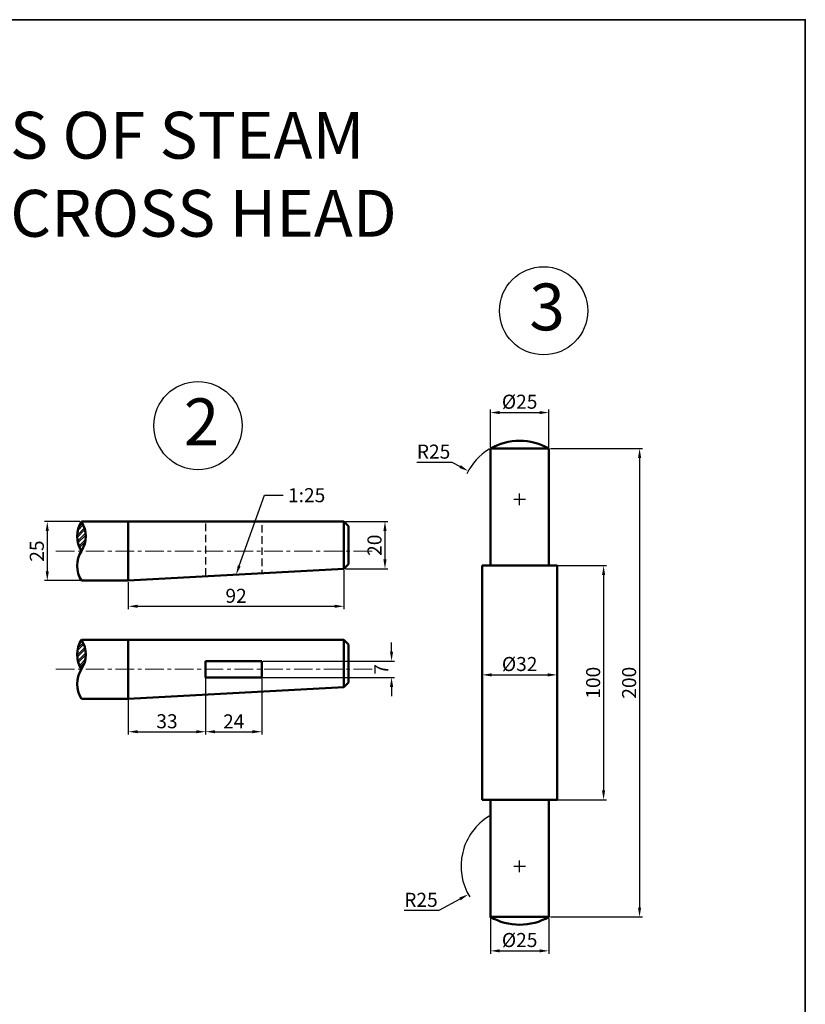
# Model space of a CAD drawing. Units: millimetres. Extents: x 208 to 901, y -26 to 704.
# Tile 3 of 3: x 566 to 901, y 283 to 704. Entities that reach past the tile are written whole.
import ezdxf
from ezdxf import colors
from ezdxf.entities.mleader import LeaderData, LeaderLine
from ezdxf.math import Vec2, Vec3

# ---------------------------------------------------------------- set-up
doc = ezdxf.new("R2010")
doc.units = ezdxf.units.MM
doc.header["$LTSCALE"] = 0.5
doc.linetypes.add('CENTER', pattern=[50.8, 31.75, -6.35, 6.35, -6.35])
doc.linetypes.add('DASHED', pattern=[19.05, 12.7, -6.35])
for name, color, linetype, lineweight in [('M-CNTR', 1, 'CENTER', 18), ('M-DIMS', 2, 'Continuous', 25), ('M-HATC', 8, 'Continuous', 18), ('M-HIDN', 6, 'DASHED', 25), ('M-OUTL', 7, 'Continuous', 50), ('M-TEXT', 3, 'Continuous', 25), ('M-TTLB', 7, 'Continuous', 35)]:
    doc.layers.add(name, color=color, linetype=linetype, lineweight=lineweight)
doc.styles.get("Standard").update_dxf_attribs({"font": 'arial.ttf'})
doc.dimstyles.new('ISO-25', dxfattribs={"dimtxt": 6, "dimasz": 4, "dimexe": 1.25, "dimexo": 0.625, "dimtad": 1, "dimtoh": 1, "dimdec": 0, "dimtxsty": 'Standard', "dimcen": 2.5, "dimadec": 0, "dimazin": 0, "dimtfac": 1, "dimtdec": 0, "dimtofl": 0, "dimtmove": 0, "dimatfit": 3, "dimfxl": 1, "dimarcsym": 0})

# ---------------------------------------------------------------- blocks, each defined once
blk = doc.blocks.new('*D32')
at = {"layer": 'Defpoints', "color": 0, "ltscale": 0.5, "transparency": 16777216}
for p in [(757.07, 510.97), (778.98, 498.94)]:
    blk.add_point(p, dxfattribs=at)
at = {"layer": 'M-DIMS', "color": 0, "lineweight": -2, "ltscale": 0.5, "transparency": 16777216}
for p, q in [((735.05, 514.83), (750.06, 514.83)), ((750.06, 514.83), (753.56, 512.9)), ((778.98, 496.44), (778.98, 501.44)), ((776.48, 498.94), (781.48, 498.94))]:
    blk.add_line(p, q, dxfattribs=at)
blk.add_arc((778.98, 498.94), 25, 121.4324, 154.0897, dxfattribs=at)
at = {"layer": 'M-DIMS', "color": 0, "ltscale": 0.5, "transparency": 16777216}
blk.add_solid([(753.88, 513.48), (753.24, 512.32), (757.07, 510.97)], dxfattribs=at)
at = {"layer": 'M-DIMS', "color": 0, "ltscale": 0.5, "transparency": 16777216, "insert": (742.24, 518.51), "char_height": 6, "attachment_point": 5}
blk.add_mtext('R25', dxfattribs=at)
blk = doc.blocks.new('*D33')
at = {"layer": 'Defpoints', "color": 0, "ltscale": 0.5, "transparency": 16777216}
for p in [(791.48, 470.59), (791.48, 370.59), (814.8, 370.59)]:
    blk.add_point(p, dxfattribs=at)
at = {"layer": 'M-DIMS', "color": 0, "lineweight": -2, "ltscale": 0.5, "transparency": 16777216}
for p, q in [((792.11, 470.59), (816.05, 470.59)), ((814.8, 466.59), (814.8, 374.59)), ((792.11, 370.59), (816.05, 370.59))]:
    blk.add_line(p, q, dxfattribs=at)
at = {"layer": 'M-DIMS', "color": 0, "ltscale": 0.5, "transparency": 16777216}
for points in [[(814.13, 466.59), (815.47, 466.59), (814.8, 470.59)], [(814.13, 374.59), (815.47, 374.59), (814.8, 370.59)]]:
    blk.add_solid(points, dxfattribs=at)
at = {"layer": 'M-DIMS', "color": 0, "ltscale": 0.5, "transparency": 16777216, "insert": (811.11, 420.59), "char_height": 6, "attachment_point": 5, "rotation": 90}
blk.add_mtext('100', dxfattribs=at)
blk = doc.blocks.new('*D34')
at = {"layer": 'Defpoints', "color": 0, "ltscale": 0.5, "transparency": 16777216}
for p in [(778.98, 342.24), (757.07, 330.21)]:
    blk.add_point(p, dxfattribs=at)
at = {"layer": 'M-DIMS', "color": 0, "lineweight": -2, "ltscale": 0.5, "transparency": 16777216}
for p, q in [((776.48, 342.24), (781.48, 342.24)), ((778.98, 339.74), (778.98, 344.74)), ((744.69, 323.41), (753.56, 328.28)), ((729.68, 323.41), (744.69, 323.41))]:
    blk.add_line(p, q, dxfattribs=at)
blk.add_arc((778.98, 342.24), 25, 121.4324, 211.6398, dxfattribs=at)
at = {"layer": 'M-DIMS', "color": 0, "ltscale": 0.5, "transparency": 16777216}
blk.add_solid([(753.24, 328.87), (753.88, 327.7), (757.07, 330.21)], dxfattribs=at)
at = {"layer": 'M-DIMS', "color": 0, "ltscale": 0.5, "transparency": 16777216, "insert": (736.87, 327.1), "char_height": 6, "attachment_point": 5}
blk.add_mtext('R25', dxfattribs=at)
blk = doc.blocks.new('*D35')
at = {"layer": 'Defpoints', "color": 0, "ltscale": 0.5, "transparency": 16777216}
for p in [(791.48, 520.59), (791.48, 320.59), (830.15, 320.59)]:
    blk.add_point(p, dxfattribs=at)
at = {"layer": 'M-DIMS', "color": 0, "lineweight": -2, "ltscale": 0.5, "transparency": 16777216}
for p, q in [((792.11, 520.59), (831.4, 520.59)), ((830.15, 516.59), (830.15, 324.59)), ((792.11, 320.59), (831.4, 320.59))]:
    blk.add_line(p, q, dxfattribs=at)
at = {"layer": 'M-DIMS', "color": 0, "ltscale": 0.5, "transparency": 16777216}
for points in [[(829.48, 516.59), (830.82, 516.59), (830.15, 520.59)], [(829.48, 324.59), (830.82, 324.59), (830.15, 320.59)]]:
    blk.add_solid(points, dxfattribs=at)
at = {"layer": 'M-DIMS', "color": 0, "ltscale": 0.5, "transparency": 16777216, "insert": (826.46, 420.59), "char_height": 6, "attachment_point": 5, "rotation": 90}
blk.add_mtext('200', dxfattribs=at)
blk = doc.blocks.new('*D36')
at = {"layer": 'Defpoints', "color": 0, "ltscale": 0.5, "transparency": 16777216}
for p in [(762.98, 420.59), (794.98, 423.96), (794.98, 420.59)]:
    blk.add_point(p, dxfattribs=at)
at = {"layer": 'M-DIMS', "color": 0, "lineweight": -2, "ltscale": 0.5, "transparency": 16777216}
for p, q in [((762.98, 421.22), (762.98, 425.21)), ((794.98, 421.22), (794.98, 425.21)), ((766.98, 423.96), (790.98, 423.96))]:
    blk.add_line(p, q, dxfattribs=at)
at = {"layer": 'M-DIMS', "color": 0, "ltscale": 0.5, "transparency": 16777216}
for points in [[(766.98, 424.62), (766.98, 423.29), (762.98, 423.96)], [(790.98, 424.62), (790.98, 423.29), (794.98, 423.96)]]:
    blk.add_solid(points, dxfattribs=at)
at = {"layer": 'M-DIMS', "color": 0, "ltscale": 0.5, "transparency": 16777216, "insert": (778.98, 427.81), "char_height": 6, "attachment_point": 5}
blk.add_mtext('%%C32', dxfattribs=at)
blk = doc.blocks.new('*D37')
at = {"layer": 'Defpoints', "color": 0, "ltscale": 0.5, "transparency": 16777216}
for p in [(791.48, 535.96), (766.48, 520.59), (791.48, 520.59)]:
    blk.add_point(p, dxfattribs=at)
at = {"layer": 'M-DIMS', "color": 0, "lineweight": -2, "ltscale": 0.5, "transparency": 16777216}
for p, q in [((766.48, 521.22), (766.48, 537.21)), ((770.48, 535.96), (787.48, 535.96)), ((791.48, 521.22), (791.48, 537.21))]:
    blk.add_line(p, q, dxfattribs=at)
at = {"layer": 'M-DIMS', "color": 0, "ltscale": 0.5, "transparency": 16777216}
for points in [[(770.48, 536.63), (770.48, 535.29), (766.48, 535.96)], [(787.48, 536.63), (787.48, 535.29), (791.48, 535.96)]]:
    blk.add_solid(points, dxfattribs=at)
at = {"layer": 'M-DIMS', "color": 0, "ltscale": 0.5, "transparency": 16777216, "insert": (778.98, 539.82), "char_height": 6, "attachment_point": 5}
blk.add_mtext('%%C25', dxfattribs=at)
blk = doc.blocks.new('*D38')
at = {"layer": 'Defpoints', "color": 0, "ltscale": 0.5, "transparency": 16777216}
for p in [(766.48, 320.59), (791.48, 320.59), (791.48, 306.09)]:
    blk.add_point(p, dxfattribs=at)
at = {"layer": 'M-DIMS', "color": 0, "lineweight": -2, "ltscale": 0.5, "transparency": 16777216}
for p, q in [((766.48, 319.97), (766.48, 304.84)), ((791.48, 319.97), (791.48, 304.84)), ((770.48, 306.09), (787.48, 306.09))]:
    blk.add_line(p, q, dxfattribs=at)
at = {"layer": 'M-DIMS', "color": 0, "ltscale": 0.5, "transparency": 16777216}
for points in [[(770.48, 306.75), (770.48, 305.42), (766.48, 306.09)], [(787.48, 306.75), (787.48, 305.42), (791.48, 306.09)]]:
    blk.add_solid(points, dxfattribs=at)
at = {"layer": 'M-DIMS', "color": 0, "ltscale": 0.5, "transparency": 16777216, "insert": (778.98, 309.94), "char_height": 6, "attachment_point": 5}
blk.add_mtext('%%C25', dxfattribs=at)
blk = doc.blocks.new('*D39')
at = {"layer": 'Defpoints', "color": 0, "ltscale": 0.5, "transparency": 16777216}
for p in [(591.98, 489.42), (577.41, 464.22), (591.98, 464.22)]:
    blk.add_point(p, dxfattribs=at)
at = {"layer": 'M-DIMS', "color": 0, "lineweight": -2, "ltscale": 0.5, "transparency": 16777216}
for p, q in [((591.35, 489.42), (576.16, 489.42)), ((577.41, 485.42), (577.41, 468.22)), ((591.35, 464.22), (576.16, 464.22))]:
    blk.add_line(p, q, dxfattribs=at)
at = {"layer": 'M-DIMS', "color": 0, "ltscale": 0.5, "transparency": 16777216}
for points in [[(576.74, 485.42), (578.07, 485.42), (577.41, 489.42)], [(576.74, 468.22), (578.07, 468.22), (577.41, 464.22)]]:
    blk.add_solid(points, dxfattribs=at)
at = {"layer": 'M-DIMS', "color": 0, "ltscale": 0.5, "transparency": 16777216, "insert": (573.72, 476.82), "char_height": 6, "attachment_point": 5, "rotation": 90}
blk.add_mtext('25', dxfattribs=at)
blk = doc.blocks.new('*D40')
at = {"layer": 'Defpoints', "color": 0, "ltscale": 0.5, "transparency": 16777216}
for p in [(703.98, 469.22), (611.98, 464.22), (703.98, 453.24)]:
    blk.add_point(p, dxfattribs=at)
at = {"layer": 'M-DIMS', "color": 0, "lineweight": -2, "ltscale": 0.5, "transparency": 16777216}
for p, q in [((703.98, 468.6), (703.98, 451.99)), ((611.98, 463.6), (611.98, 451.99)), ((615.98, 453.24), (699.98, 453.24))]:
    blk.add_line(p, q, dxfattribs=at)
at = {"layer": 'M-DIMS', "color": 0, "ltscale": 0.5, "transparency": 16777216}
for points in [[(615.98, 453.91), (615.98, 452.57), (611.98, 453.24)], [(699.98, 453.91), (699.98, 452.57), (703.98, 453.24)]]:
    blk.add_solid(points, dxfattribs=at)
at = {"layer": 'M-DIMS', "color": 0, "ltscale": 0.5, "transparency": 16777216, "insert": (657.98, 456.93), "char_height": 6, "attachment_point": 5}
blk.add_mtext('92', dxfattribs=at)
blk = doc.blocks.new('*D41')
at = {"layer": 'Defpoints', "color": 0, "ltscale": 0.5, "transparency": 16777216}
for p in [(703.98, 489.42), (703.98, 469.22), (721.51, 469.22)]:
    blk.add_point(p, dxfattribs=at)
at = {"layer": 'M-DIMS', "color": 0, "lineweight": -2, "ltscale": 0.5, "transparency": 16777216}
for p, q in [((704.6, 489.42), (722.76, 489.42)), ((721.51, 485.42), (721.51, 473.22)), ((704.6, 469.22), (722.76, 469.22))]:
    blk.add_line(p, q, dxfattribs=at)
at = {"layer": 'M-DIMS', "color": 0, "ltscale": 0.5, "transparency": 16777216}
for points in [[(720.84, 485.42), (722.17, 485.42), (721.51, 489.42)], [(720.84, 473.22), (722.17, 473.22), (721.51, 469.22)]]:
    blk.add_solid(points, dxfattribs=at)
at = {"layer": 'M-DIMS', "color": 0, "ltscale": 0.5, "transparency": 16777216, "insert": (717.82, 479.32), "char_height": 6, "attachment_point": 5, "rotation": 90}
blk.add_mtext('20', dxfattribs=at)
blk = doc.blocks.new('*D42')
at = {"layer": 'Defpoints', "color": 0, "ltscale": 0.5, "transparency": 16777216}
for p in [(611.98, 426.33), (644.98, 426.33), (644.98, 399.67)]:
    blk.add_point(p, dxfattribs=at)
at = {"layer": 'M-DIMS', "color": 0, "lineweight": -2, "ltscale": 0.5, "transparency": 16777216}
for p, q in [((611.98, 425.71), (611.98, 398.42)), ((644.98, 425.71), (644.98, 398.42)), ((615.98, 399.67), (640.98, 399.67))]:
    blk.add_line(p, q, dxfattribs=at)
at = {"layer": 'M-DIMS', "color": 0, "ltscale": 0.5, "transparency": 16777216}
for points in [[(615.98, 400.34), (615.98, 399.01), (611.98, 399.67)], [(640.98, 400.34), (640.98, 399.01), (644.98, 399.67)]]:
    blk.add_solid(points, dxfattribs=at)
at = {"layer": 'M-DIMS', "color": 0, "ltscale": 0.5, "transparency": 16777216, "insert": (628.48, 403.36), "char_height": 6, "attachment_point": 5}
blk.add_mtext('33', dxfattribs=at)
blk = doc.blocks.new('*D43')
at = {"layer": 'Defpoints', "color": 0, "ltscale": 0.5, "transparency": 16777216}
for p in [(644.98, 426.33), (668.98, 426.33), (668.98, 399.67)]:
    blk.add_point(p, dxfattribs=at)
at = {"layer": 'M-DIMS', "color": 0, "lineweight": -2, "ltscale": 0.5, "transparency": 16777216}
for p, q in [((644.98, 425.71), (644.98, 398.42)), ((668.98, 425.71), (668.98, 398.42)), ((648.98, 399.67), (664.98, 399.67))]:
    blk.add_line(p, q, dxfattribs=at)
at = {"layer": 'M-DIMS', "color": 0, "ltscale": 0.5, "transparency": 16777216}
for points in [[(648.98, 400.34), (648.98, 399.01), (644.98, 399.67)], [(664.98, 400.34), (664.98, 399.01), (668.98, 399.67)]]:
    blk.add_solid(points, dxfattribs=at)
at = {"layer": 'M-DIMS', "color": 0, "ltscale": 0.5, "transparency": 16777216, "insert": (656.98, 403.31), "char_height": 6, "attachment_point": 5}
blk.add_mtext('24', dxfattribs=at)
blk = doc.blocks.new('*D44')
at = {"layer": 'Defpoints', "color": 0, "ltscale": 0.5, "transparency": 16777216}
for p in [(668.98, 429.83), (668.98, 422.83), (724.32, 422.83)]:
    blk.add_point(p, dxfattribs=at)
at = {"layer": 'M-DIMS', "color": 0, "lineweight": -2, "ltscale": 0.5, "transparency": 16777216}
for p, q in [((724.32, 433.83), (724.32, 437.83)), ((669.6, 429.83), (725.57, 429.83)), ((669.6, 422.83), (725.57, 422.83)), ((724.32, 418.83), (724.32, 414.83))]:
    blk.add_line(p, q, dxfattribs=at)
at = {"layer": 'M-DIMS', "color": 0, "ltscale": 0.5, "transparency": 16777216}
for points in [[(723.65, 433.83), (724.99, 433.83), (724.32, 429.83)], [(723.65, 418.83), (724.99, 418.83), (724.32, 422.83)]]:
    blk.add_solid(points, dxfattribs=at)
at = {"layer": 'M-DIMS', "color": 0, "ltscale": 0.5, "transparency": 16777216, "insert": (720.69, 426.33), "char_height": 6, "attachment_point": 5, "rotation": 90}
blk.add_mtext('7', dxfattribs=at)

msp = doc.modelspace()

# ---------------------------------------------------------------- hatches: boundary and pattern name
at = {"layer": 'M-HATC', "ltscale": 0.5}
h = msp.add_hatch(dxfattribs=at)
h.set_pattern_fill('ANSI32', color=256, scale=0.2)
h.set_pattern_definition([(45, (0.9211, 274.185), (-1.3470384, 1.3470384), []), (45, (1.8191, 274.185), (-1.3470384, 1.3470384), [])])
h.paths.add_polyline_path([(591.9798, 476.8237, 0.29492277), (591.9798, 489.4237, 0.29492277)])
h.paths.add_polyline_path([(591.9798, 438.9347, 0.29492277), (591.9798, 426.3347, 0.29492277)])

# ---------------------------------------------------------------- linework, layer by layer
at = {"layer": 'M-CNTR', "ltscale": 0.5}
for p, q in [((581.0932, 476.8237), (717.2894, 476.8237)), ((581.0932, 426.3347), (717.2894, 426.3347))]:
    msp.add_line(p, q, dxfattribs=at)
at = {"layer": 'M-HIDN', "ltscale": 0.5}
for p, q in [((644.9798, 488.527), (644.9798, 466.0172)), ((668.9798, 487.8748), (668.9798, 467.3215))]:
    msp.add_line(p, q, dxfattribs=at)
at = {"layer": 'M-OUTL', "ltscale": 0.5}
for p, q in [((766.4814, 520.5906), (766.4814, 470.5906)), ((791.4814, 470.5906), (791.4814, 520.5906)), ((611.9798, 489.4237), (591.9798, 489.4237)), ((611.9798, 489.4237), (703.9798, 489.4237)), ((611.9798, 489.4237), (611.9798, 464.2237)), ((703.9798, 489.4237), (703.9798, 469.2237)), ((703.9798, 489.4237), (705.9798, 487.4237)), ((705.9798, 487.4237), (705.9798, 471.2237)), ((703.9798, 469.2237), (705.9798, 471.2237)), ((611.9798, 464.2237), (703.9798, 469.2237)), ((762.9814, 470.5906), (794.9814, 470.5906)), ((762.9814, 370.5906), (762.9814, 470.5906)), ((791.4814, 470.5906), (766.4814, 470.5906)), ((794.9814, 470.5906), (794.9814, 370.5906)), ((611.9798, 464.2237), (591.9798, 464.2237)), ((611.9798, 438.9347), (591.9798, 438.9347)), ((611.9798, 438.9347), (703.9798, 438.9347)), ((611.9798, 438.9347), (611.9798, 413.7347)), ((703.9798, 438.9347), (703.9798, 418.7347)), ((703.9798, 438.9347), (705.9798, 436.9347)), ((705.9798, 436.9347), (705.9798, 420.7347)), ((644.9798, 429.8347), (668.9798, 429.8347)), ((644.9798, 422.8347), (644.9798, 429.8347)), ((668.9798, 429.8347), (668.9798, 422.8347)), ((668.9798, 422.8347), (644.9798, 422.8347)), ((703.9798, 418.7347), (705.9798, 420.7347)), ((611.9798, 413.7347), (703.9798, 418.7347)), ((611.9798, 413.7347), (591.9798, 413.7347)), ((794.9814, 370.5906), (762.9814, 370.5906)), ((766.4814, 320.5906), (766.4814, 370.5906)), ((791.4814, 370.5906), (766.4814, 370.5906)), ((791.4814, 370.5906), (791.4814, 320.5906))]:
    msp.add_line(p, q, dxfattribs=at)
for points in [[(791.4814, 520.5906, 0.26794919), (766.4814, 520.5906)], [(791.4814, 320.5906, -0.26794919), (766.4814, 320.5906)]]:
    msp.add_lwpolyline(points, format="xyb", close=True, dxfattribs=at)
for centre, start, end in [((601.7315, 483.1237), 147.136024, 212.863976), ((582.228, 483.1237), 327.136024, 32.863976), ((601.7315, 470.5237), 147.136024, 212.863976), ((601.7315, 432.6347), 147.136024, 212.863976), ((582.228, 432.6347), 327.136024, 32.863976), ((601.7315, 420.0347), 147.136024, 212.863976)]:
    msp.add_arc(centre, 11.6098, start, end, dxfattribs=at)
at = {"layer": 'M-TEXT', "ltscale": 0.5}
for centre in [(789.1847, 579.4341), (641.7109, 530.3797)]:
    msp.add_circle(centre, 18.8257, dxfattribs=at)
at = {"layer": 'M-TTLB', "ltscale": 0.5}
msp.add_lwpolyline([(208.2585, 703.7432), (900.8689, 703.7432), (900.8689, -25.914), (208.2585, -25.914)], close=True, dxfattribs=at)

# ---------------------------------------------------------------- texts
at = {"layer": 'M-TEXT', "ltscale": 0.5, "char_height": 20, "attachment_point": 1}
for s, width, insert in [('\\pxqc;DETAILS OF STEAM ENGINE CROSS HEAD', 309.964733, (436.8417, 664.3913)), ('3', 20, (783.1289, 591.0701)), ('2', 20, (635.6551, 542.0158))]:
    msp.add_mtext_dynamic_manual_height_columns(s, width=width, gutter_width=12.5, heights=[0], dxfattribs=dict(at, insert=insert))

# ---------------------------------------------------------------- dimensions: what is measured, and where the dimension line sits
at = {"layer": 'M-DIMS', "ltscale": 0.5}
for base, p1, p2, picture, middle in [((791.4814, 535.96), (766.4814, 520.5906), (791.4814, 520.5906), '*D37', (778.9814, 539.8163)), ((794.9814, 423.9569), (762.9814, 420.5906), (794.9814, 420.5906), '*D36', (778.9814, 427.8132)), ((791.4814, 306.088), (766.4814, 320.5906), (791.4814, 320.5906), '*D38', (778.9814, 309.9443))]:
    dim = msp.add_linear_dim(base=base, p1=p1, p2=p2, text='%%C<>', dimstyle='ISO-25', override={"dimclrd": 0, "dimclre": 0, "dimclrt": 0}, dxfattribs=at)
    dim.commit()
    dim.dimension.update_dxf_attribs({"geometry": picture, "text_midpoint": middle})
for center, mpoint, picture, middle in [((778.9814, 498.9399), (757.0685, 510.9742), '*D32', (742.2403, 518.5136)), ((778.9814, 342.2412), (757.0685, 330.2069), '*D34', (736.87, 327.0951))]:
    dim = msp.add_radius_dim(center=center, mpoint=mpoint, dimstyle='ISO-25', override={"dimclrd": 0, "dimclre": 0, "dimclrt": 0}, dxfattribs=at)
    dim.commit()
    dim.dimension.update_dxf_attribs({"geometry": picture, "text_midpoint": middle})
for base, p1, p2, picture, middle in [((830.1511, 320.5906), (791.4814, 520.5906), (791.4814, 320.5906), '*D35', (826.4627, 420.5906)), ((577.4073, 464.2237), (591.9798, 489.4237), (591.9798, 464.2237), '*D39', (573.7189, 476.8237)), ((814.8001, 370.5906), (791.4814, 470.5906), (791.4814, 370.5906), '*D33', (811.1117, 420.5906)), ((724.3186, 422.8347), (668.9798, 429.8347), (668.9798, 422.8347), '*D44', (720.6936, 426.3347))]:
    dim = msp.add_linear_dim(base=base, p1=p1, p2=p2, angle=90, dimstyle='ISO-25', override={"dimclrd": 0, "dimclre": 0, "dimclrt": 0}, dxfattribs=at)
    dim.commit()
    dim.dimension.update_dxf_attribs({"geometry": picture, "text_midpoint": middle})
dim = msp.add_linear_dim(base=(721.5058, 469.2237), p1=(703.9798, 489.4237), p2=(703.9798, 469.2237), angle=90, dimstyle='ISO-25', override={"dimclrd": 0, "dimclre": 0, "dimclrt": 0}, dxfattribs=at)
dim.commit()
dim.dimension.update_dxf_attribs({"geometry": '*D41', "text_midpoint": (721.5058, 479.3237), "dimtype": 160})
for base, p1, p2, picture, middle in [((703.9798, 453.2397), (611.9798, 464.2237), (703.9798, 469.2237), '*D40', (657.9798, 456.9282)), ((644.9798, 399.6737), (611.9798, 426.3347), (644.9798, 426.3347), '*D42', (628.4798, 403.3642)), ((668.9798, 399.6737), (644.9798, 426.3347), (668.9798, 426.3347), '*D43', (656.9798, 403.3109))]:
    dim = msp.add_linear_dim(base=base, p1=p1, p2=p2, dimstyle='ISO-25', override={"dimclrd": 0, "dimclre": 0, "dimclrt": 0}, dxfattribs=at)
    dim.commit()
    dim.dimension.update_dxf_attribs({"geometry": picture, "text_midpoint": middle})

# ---------------------------------------------------------------- leaders
ml = msp.add_multileader_mtext('Standard', dxfattribs=at)
ml.set_content('1:25', color=256)
ml.set_leader_properties()
ml.build(insert=Vec2(0, 0))
ctx = ml.context
ctx.base_point, ctx.char_height, ctx.plane_origin = Vec3(678.1374, 500.6234), 6, Vec3(658.5776, 467.3215)
notes = []
notes.append((ctx, [(0, (1, 1, 0), (670.1374, 500.6234), (1, 0), 8, [(0, [(657.9798, 466.7237)], 0, [])])]))
ctx.mtext.insert, ctx.mtext.flow_direction = Vec3(680.1374, 503.6746), 5
for ctx, leaders in notes:
    for number, flags, end, landing, length, lines in leaders:
        leader = LeaderData()
        leader.index, (leader.has_last_leader_line, leader.has_dogleg_vector, leader.attachment_direction) = number, flags
        leader.last_leader_point, leader.dogleg_vector, leader.dogleg_length = Vec3(end), Vec3(landing), length
        for number, points, colour, breaks in lines:
            line = LeaderLine()
            line.index, line.vertices, line.color, line.breaks = number, Vec3.list(points), colors.encode_raw_color(colour), breaks
            leader.lines.append(line)
        ctx.leaders.append(leader)

doc.saveas('drawing.dxf')
